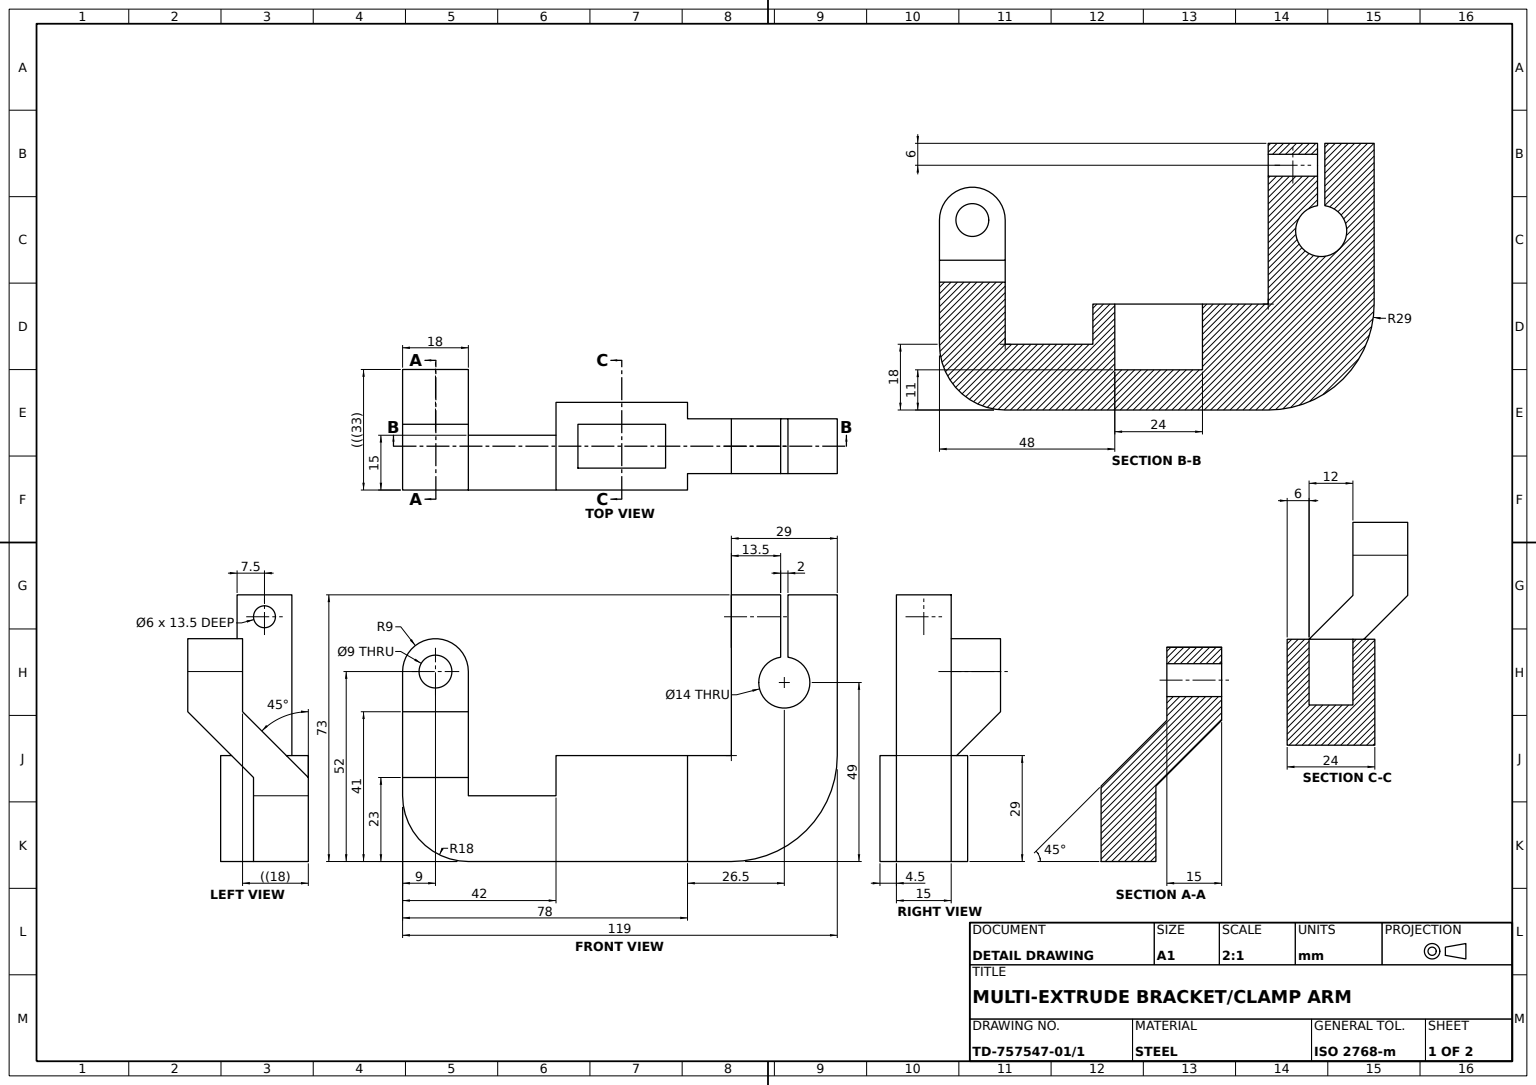
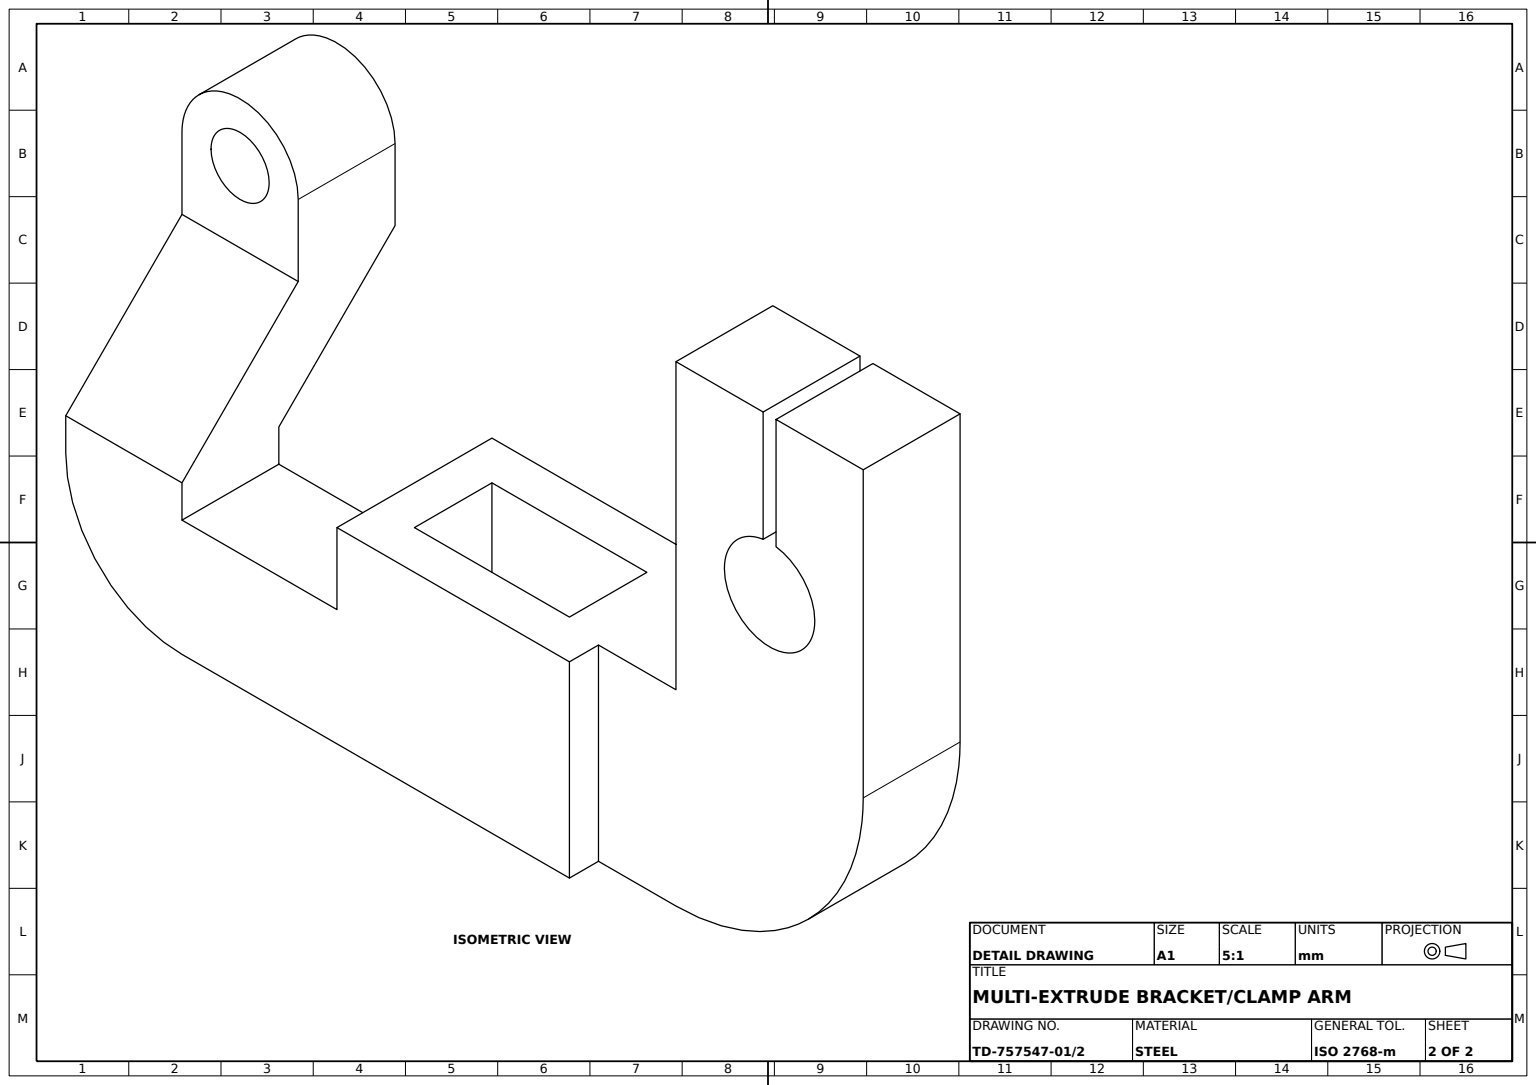
SolidWorks part; units mm, degrees
material "Plain Carbon Steel"
ref_plane "Front Plane" through (0, 0, 0) normal (0, 0, 1) x (1, 0, 0)
ref_plane "Top Plane" through (0, 0, 0) normal (0, 1, 0) x (1, 0, 0)
ref_plane "Right Plane" through (0, 0, 0) normal (1, 0, 0) x (0, 0, -1)
sketch "Base Profile Sketch" plane through (0, 0, 0) normal (0, 0, 1) x (1, 0, 0)
  line L0 (0, -18) -> (60, -18)
  line L1 (60, -18) -> (60, 11)
  line L2 (-18, 0) -> (-18, 5)
  line L3 (-18, 5) -> (0, 5)
  line L4 (0, 5) -> (0, 0)
  line L5 (0, 0) -> (24, 0)
  line L6 (24, 0) -> (24, 11)
  line L7 (24, 11) -> (60, 11)
  arc A0 (-18, 0) -> (0, -18) centre (0, 0) ccw
  dimension "D1" = 18
  dimension "D2" = 42
  dimension "D3" = 78
  dimension "D4" = 23
  dimension "D5" = 29
extrude "Base Body" add sketch "Base Profile Sketch" along normal blind 15
sketch "Arm Block Sketch" plane through (-18, 0, 0) normal (-1, 0, 0) x (0, 0, 1)
  line L0 (0, 5) -> (0, 0) construction
  line L1 (15, 0) -> (0, 0) construction
  line L2 (-18, 23) -> (-3, 23)
  line L3 (-3, 23) -> (15, 5)
  line L4 (15, 5) -> (0, 5)
  line L5 (0, 5) -> (-18, 23)
  dimension "D1" = 3
  dimension "D2" = 23
extrude "Arm Block" add sketch "Arm Block Sketch" against normal blind 18
sketch "Inclined Arm Sketch" plane through (-18, 0, 0) normal (-1, 0, 0) x (0, 0, 1)
  line L0 (-18, 23) -> (-18, 34)
  line L1 (-18, 34) -> (-3, 34)
  line L2 (-3, 34) -> (-3, 23)
  line L3 (-3, 23) -> (-18, 23)
  line L5 (15, 0) -> (0, 0) construction
  dimension "D1" = 34
extrude "Inclined Arm" add sketch "Inclined Arm Sketch" against normal blind 18
sketch "Top Lug Sketch" plane through (0, 0, -3) normal (0, 0, 1) x (1, 0, 0)
  line L0 (0, 34) -> (-18, 34) construction
  line L1 (-18, 34) -> (0, 34)
  arc A0 (0, 34) -> (-18, 34) centre (-9, 34) ccw
  dimension "D1" = 18
extrude "Top Lug" add sketch "Top Lug Sketch" against normal blind 15
sketch "Lug Hole Sketch" plane through (0, 0, -3) normal (0, 0, 1) x (1, 0, 0)
  circle A0 centre (-9, 34) radius 4.5
  dimension "D1" = 9
  dimension "D2" = 9
extrude "Lug Hole Ø9" cut sketch "Lug Hole Sketch" against normal blind 15
sketch "Pocket Boss Sketch" plane through (0, 0, 0) normal (0, 0, -1) x (-1, 0, 0)
  line L0 (-60, 11) -> (-24, 11)
  line L1 (-24, 11) -> (-24, -18)
  line L2 (0, -18) -> (-60, -18) construction
  line L3 (-24, -18) -> (-60, -18)
  line L4 (-60, -18) -> (-60, 11)
extrude "Pocket Boss" add sketch "Pocket Boss Sketch" along normal blind 9
sketch "Clevis Block Sketch" plane through (0, 11, 0) normal (0, 1, 0) x (1, 0, 0)
  line L0 (24, 9) -> (60, 9) construction
  line L1 (60, -15) -> (60, 9) construction
  line L2 (60, 4.5) -> (72, 4.5)
  line L3 (72, 4.5) -> (72, -10.5)
  line L4 (72, -10.5) -> (60, -10.5)
  line L6 (60, -10.5) -> (60, 4.5)
  dimension "D1" = 12
  dimension "D2" = 4.5
  dimension "D3" = 19.5
extrude "Clevis Block" add sketch "Clevis Block Sketch" against normal blind 29
sketch "Clevis Corner Sketch" plane through (0, 0, 10.5) normal (0, 0, 1) x (1, 0, 0)
  line L0 (72, 11) -> (101, 11)
  line L1 (72, 11) -> (72, -18)
  arc A0 (72, -18) -> (101, 11) centre (72, 11) ccw
  dimension "D1" = 29
extrude "Clevis Corner" add sketch "Clevis Corner Sketch" against normal blind 15
sketch "Clevis Jaw Sketch" plane through (0, 0, 10.5) normal (0, 0, 1) x (1, 0, 0)
  line L0 (101, 11) -> (72, 11)
  line L1 (72, 11) -> (72, 31)
  line L2 (72, 31) -> (72, 55)
  line L3 (72, 55) -> (101, 55)
  line L4 (101, 55) -> (101, 11)
  line L6 (60, 11) -> (101, 11) construction
  dimension "D1" = 20
  dimension "D2" = 44
extrude "Clevis Jaw" add sketch "Clevis Jaw Sketch" against normal blind 15
sketch "Clevis Hole Sketch" plane through (0, 0, 10.5) normal (0, 0, 1) x (1, 0, 0)
  line L0 (60, -18) -> (60, 11) construction
  line L1 (60, -18) -> (72, -18) construction
  circle A0 centre (86.5, 31) radius 7
  dimension "D1" = 14
  dimension "D2" = 14
  dimension "D3" = 26.5
  dimension "D4" = 49
extrude "Clevis Hole Ø14" cut sketch "Clevis Hole Sketch" against normal blind 15
sketch "Clevis Slot Sketch" plane through (0, 55, 0) normal (0, 1, 0) x (1, 0, 0)
  line L0 (86.5, 4.5) -> (85.5, 4.5)
  line L1 (101, 4.5) -> (72, 4.5) construction
  line L2 (85.5, 4.5) -> (85.5, -10.5)
  line L3 (101, 4.5) -> (101, -10.5) construction
  line L4 (85.5, -10.5) -> (87.5, -10.5)
  line L5 (101, -10.5) -> (72, -10.5) construction
  line L6 (87.5, -10.5) -> (87.5, 4.5)
  line L7 (87.5, 4.5) -> (86.5, 4.5)
  dimension "D1" = 13.5
extrude "Clevis Slot" cut sketch "Clevis Slot Sketch" against normal blind 18
sketch "Jaw Hole Sketch" plane through (72, 0, 0) normal (-1, 0, 0) x (0, 0, 1)
  line L0 (-4.5, 55) -> (10.5, 55) construction
  line L1 (10.5, 55) -> (10.5, 11) construction
  circle A0 centre (3, 49) radius 3
  dimension "D1" = 6
  dimension "D3" = 6
  dimension "D2" = 6
  dimension "D4" = 7.5
extrude "Jaw Hole Ø6" cut sketch "Jaw Hole Sketch" against normal blind 15
sketch "Rectangular Pocket Sketch" plane through (0, 11, 0) normal (0, 1, 0) x (1, 0, 0)
  line L0 (60, -15) -> (24, -15) construction
  line L1 (30, 3) -> (54, 3)
  line L2 (30, 3) -> (30, -9)
  line L3 (30, -9) -> (54, -9)
  line L4 (54, 3) -> (54, -9)
  line L5 (24, 9) -> (60, 9) construction
  line L6 (24, -15) -> (24, 9) construction
  dimension "D1" = 24
  dimension "D2" = 6
  dimension "D3" = 6
  dimension "D4" = 6
extrude "Rectangular Pocket" cut sketch "Rectangular Pocket Sketch" against normal blind 18
